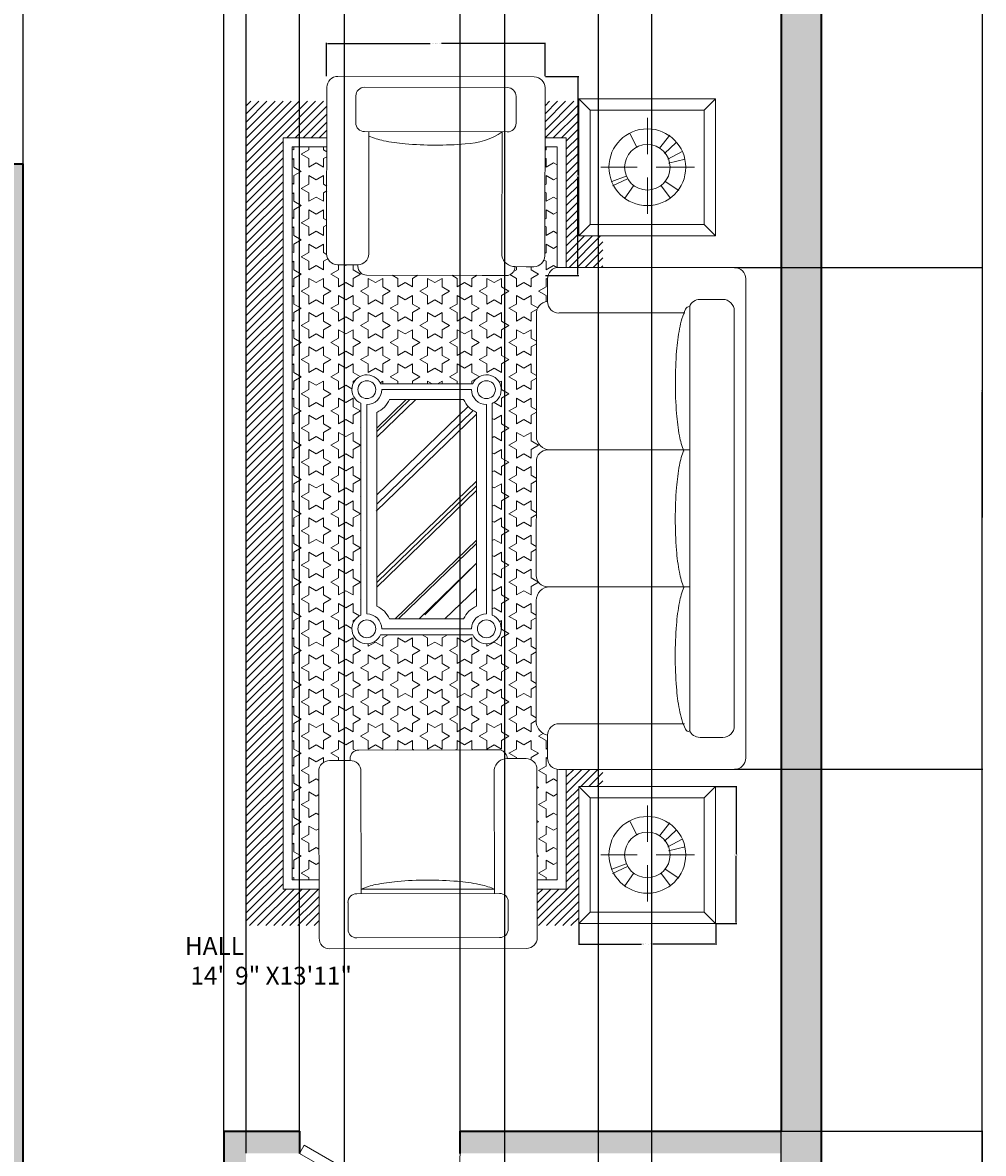
# Model space of a CAD drawing. Units: inches. Extents: x -29 to 404, y -32 to 761.
# Tile 4 of 5: x 189 to 404, y 193 to 447. Entities that reach past the tile are written whole.
import ezdxf

# ---------------------------------------------------------------- set-up
doc = ezdxf.new("R2010")
doc.units = ezdxf.units.IN
doc.header["$MEASUREMENT"] = 0
for name, color, linetype, lineweight in [('A-ANNO-DIMS', 2, 'Continuous', 18), ('A-AREA-IDEN', 7, 'Continuous', 18), ('A-FLOR-PATT', 9, 'Continuous', 13), ('A-FURN', 8, 'Continuous', 18), ('A-WALL', 7, 'Continuous', 35), ('doors', 40, 'Continuous', 20)]:
    doc.layers.add(name, color=color, linetype=linetype, lineweight=lineweight)
doc.layers.add('A-WALL-PATT', color=251, linetype='Continuous', lineweight=13, true_color=0x636466)
doc.styles.get("Standard").update_dxf_attribs({"font": 'arial.ttf'})
doc.dimstyles.get("Standard").update_dxf_attribs({"dimtxt": 0.18, "dimasz": 0.18, "dimexe": 0.18, "dimexo": 0.0625, "dimgap": 0.09, "dimtad": 0, "dimtih": 1, "dimtoh": 1, "dimdec": 4, "dimzin": 0, "dimdsep": 46, "dimtxsty": 'Standard', "dimcen": 0.09, "dimadec": 0, "dimazin": 0, "dimtfac": 1, "dimtdec": 4, "dimtofl": 0, "dimtmove": 0, "dimatfit": 3, "dimfxl": 1, "dimtolj": 1, "dimtzin": 0, "dimarcsym": 0})
pattern_1 = [(45, (602.1246, 1762.0968), (0.9050907, -0.9050907), [])]

# ---------------------------------------------------------------- blocks, each defined once
blk = doc.blocks.new('*U7')
for p, q in [((0, 0), (0, 100)), ((750, 0), (750, 100))]:
    blk.add_line(p, q)
blk.add_lwpolyline([(0, 0), (649.5, -375), (671.4, -337.1), (21.9, 37.9)], close=True)
blk.add_arc((0, 0), 750, 330, 0)
blk = doc.blocks.new('END-TABLE-HALL')
for p, q in [((0, 0), (0, 30.72)), ((0, 30.72), (30.72, 30.72)), ((2.56, 28.16), (0, 30.72)), ((28.16, 28.16), (30.72, 30.72)), ((30.72, 30.72), (30.72, 0)), ((2.56, 28.16), (28.16, 28.16)), ((2.56, 2.56), (2.56, 28.16)), ((28.16, 28.16), (28.16, 2.56)), ((15.4, 18.29), (15.4, 26.44)), ((12.94, 19.98), (11.56, 22.9)), ((18.16, 19.68), (20.47, 22.6)), ((19.24, 18.45), (21.85, 20.91)), ((20.01, 17.22), (23.23, 18.91)), ((4.95, 15.38), (13.09, 15.38)), ((17.4, 15.38), (26, 15.38)), ((20.16, 16.3), (23.85, 17.22)), ((10.64, 13.38), (7.41, 12.15)), ((10.94, 12.77), (7.56, 11.23)), ((15.4, 4.93), (15.4, 13.07)), ((12.33, 11.23), (10.33, 8.46)), ((18.47, 11.23), (20.62, 8.46)), ((19.39, 12.15), (22.46, 10.15)), ((2.56, 2.56), (0, 0)), ((28.16, 2.56), (2.56, 2.56)), ((28.16, 2.56), (30.72, 0)), ((30.72, 0), (0, 0))]:
    blk.add_line(p, q)
for radius in [8.61, 5.11]:
    blk.add_circle((15.4, 15.38), radius)
blk = doc.blocks.new('ARMCHAIR-HALL')
for p, q in [((8.97, 44.58), (35.98, 44.64)), ((34.86, 44.63), (40.72, 44.64)), ((2.43, 42.25), (7.02, 42.26)), ((7.02, 42.26), (7.03, 42.63)), ((44.98, 42.69), (42.28, 42.68)), ((44.74, 42.7), (46.49, 42.7)), ((0.07, 2.43), (0, 39.82)), ((9.51, 12.37), (9.46, 39.84)), ((39.38, 12.44), (39.33, 40.24)), ((49.01, 2.54), (48.93, 40.28)), ((6.56, 10.42), (6.57, 4.39)), ((8.5, 12.37), (40.53, 12.44)), ((42.49, 4.47), (42.48, 10.5)), ((2.51, 0), (46.58, 0.1)), ((8.52, 2.44), (40.55, 2.52))]:
    blk.add_line(p, q)
for centre, radius, start, end in [((8.97, 42.64), 1.95, 90.1148, 180.1148), ((40.17, 42.59), 2.11, 2.3345, 74.9758), ((2.43, 39.82), 2.43, 90.1148, 180.1148), ((7.03, 39.83), 2.43, 0.1148, 90.1148), ((42.21, 39.75), 2.93, 88.725, 170.3573), ((46.5, 40.27), 2.43, 0.1148, 90.1148), ((8.5, 10.42), 1.95, 90.1148, 180.1148), ((40.54, 10.5), 1.95, 0.1148, 90.1148), ((8.51, 4.39), 1.95, 180.1148, 270.1148), ((40.55, 4.47), 1.95, 270.1148, 0.1148), ((46.57, 2.53), 2.43, 270.1148, 0.1148), ((2.51, 2.43), 2.43, 180.1148, 270.1298)]:
    blk.add_arc(centre, radius, start, end)
blk = doc.blocks.new('*D17')
at = {"layer": 'A-ANNO-DIMS', "color": 0, "lineweight": -2, "transparency": 16777216}
for p, q in [((313.28, 244.96), (313.28, 240.23)), ((344, 244.96), (344, 240.23)), ((313.46, 240.41), (327.38, 240.41)), ((343.82, 240.41), (329.89, 240.41))]:
    blk.add_line(p, q, dxfattribs=at)
at = {"layer": 'A-ANNO-DIMS', "color": 0, "transparency": 16777216}
for points in [[(313.46, 240.44), (313.46, 240.38), (313.28, 240.41)], [(343.82, 240.44), (343.82, 240.38), (344, 240.41)]]:
    blk.add_solid(points, dxfattribs=at)
at = {"layer": 'Defpoints', "color": 0, "transparency": 16777216}
for p in [(313.28, 245.02), (344, 245.02), (344, 240.41)]:
    blk.add_point(p, dxfattribs=at)
at = {"layer": 'A-ANNO-DIMS', "color": 0, "transparency": 16777216, "insert": (328.64, 240.41), "char_height": 0.18, "attachment_point": 5}
blk.add_mtext('\\A1;END TABLE 31 TYP.', dxfattribs=at)
blk = doc.blocks.new('*D18')
at = {"layer": 'A-ANNO-DIMS', "color": 0, "lineweight": -2, "transparency": 16777216}
for p, q in [((344.06, 275.74), (348.78, 275.74)), ((348.6, 275.56), (348.6, 260.56)), ((348.6, 245.2), (348.6, 260.2)), ((344.06, 245.02), (348.78, 245.02))]:
    blk.add_line(p, q, dxfattribs=at)
at = {"layer": 'A-ANNO-DIMS', "color": 0, "transparency": 16777216}
for points in [[(348.57, 275.56), (348.63, 275.56), (348.6, 275.74)], [(348.57, 245.2), (348.63, 245.2), (348.6, 245.02)]]:
    blk.add_solid(points, dxfattribs=at)
at = {"layer": 'Defpoints', "color": 0, "transparency": 16777216}
for p in [(344, 275.74), (348.6, 275.74), (344, 245.02)]:
    blk.add_point(p, dxfattribs=at)
at = {"layer": 'A-ANNO-DIMS', "color": 0, "transparency": 16777216, "insert": (348.6, 260.38), "char_height": 0.18, "attachment_point": 5}
blk.add_mtext('\\A1;31 TYP.', dxfattribs=at)
blk = doc.blocks.new('*D21')
at = {"layer": 'A-ANNO-DIMS', "color": 0, "lineweight": -2, "transparency": 16777216}
for p, q in [((256.74, 435.12), (256.74, 442.59)), ((256.92, 442.41), (280.01, 442.41)), ((305.57, 442.41), (282.48, 442.41)), ((305.75, 435.12), (305.75, 442.59))]:
    blk.add_line(p, q, dxfattribs=at)
at = {"layer": 'A-ANNO-DIMS', "color": 0, "transparency": 16777216}
for points in [[(256.92, 442.44), (256.92, 442.38), (256.74, 442.41)], [(305.57, 442.44), (305.57, 442.38), (305.75, 442.41)]]:
    blk.add_solid(points, dxfattribs=at)
at = {"layer": 'Defpoints', "color": 0, "transparency": 16777216}
for p in [(305.75, 442.41), (256.74, 435.06), (305.75, 435.06)]:
    blk.add_point(p, dxfattribs=at)
at = {"layer": 'A-ANNO-DIMS', "color": 0, "transparency": 16777216, "insert": (281.25, 442.41), "char_height": 0.18, "attachment_point": 5}
blk.add_mtext('\\A1;ARMCHAIR 49 TYP.', dxfattribs=at)
blk = doc.blocks.new('*D22')
at = {"layer": 'A-ANNO-DIMS', "color": 0, "lineweight": -2, "transparency": 16777216}
for p, q in [((305.81, 435.06), (313.28, 435.06)), ((313.1, 434.88), (313.1, 412.92)), ((313.1, 390.6), (313.1, 412.56)), ((305.81, 390.42), (313.28, 390.42))]:
    blk.add_line(p, q, dxfattribs=at)
at = {"layer": 'A-ANNO-DIMS', "color": 0, "transparency": 16777216}
for points in [[(313.07, 434.88), (313.13, 434.88), (313.1, 435.06)], [(313.07, 390.6), (313.13, 390.6), (313.1, 390.42)]]:
    blk.add_solid(points, dxfattribs=at)
at = {"layer": 'Defpoints', "color": 0, "transparency": 16777216}
for p in [(305.75, 435.06), (305.75, 390.42), (313.1, 390.42)]:
    blk.add_point(p, dxfattribs=at)
at = {"layer": 'A-ANNO-DIMS', "color": 0, "transparency": 16777216, "insert": (313.1, 412.74), "char_height": 0.18, "attachment_point": 5}
blk.add_mtext('\\A1;45 TYP.', dxfattribs=at)
blk = doc.blocks.new('*D32')
at = {"layer": 'A-ANNO-DIMS', "color": 0, "lineweight": -2, "transparency": 16777216}
for p, q in [((367.74, 724.43), (403.91, 724.43)), ((403.73, 724.25), (403.73, 364.62)), ((403.73, 4.61), (403.73, 364.25)), ((367.74, 4.43), (403.91, 4.43))]:
    blk.add_line(p, q, dxfattribs=at)
at = {"layer": 'A-ANNO-DIMS', "color": 0, "transparency": 16777216}
for points in [[(403.7, 724.25), (403.76, 724.25), (403.73, 724.43)], [(403.7, 4.61), (403.76, 4.61), (403.73, 4.43)]]:
    blk.add_solid(points, dxfattribs=at)
at = {"layer": 'Defpoints', "color": 0, "transparency": 16777216}
for p in [(367.68, 724.43), (403.73, 724.43), (367.68, 4.43)]:
    blk.add_point(p, dxfattribs=at)
at = {"layer": 'A-ANNO-DIMS', "color": 0, "transparency": 16777216, "insert": (403.73, 364.43), "char_height": 0.18, "attachment_point": 5}
blk.add_mtext('\\A1;720', dxfattribs=at)
blk = doc.blocks.new('*D41')
at = {"layer": 'A-ANNO-DIMS', "color": 0, "lineweight": -2, "transparency": 16777216}
for p, q in [((250.68, 193.5), (250.68, 760.66)), ((250.86, 760.48), (268.46, 760.48)), ((286.5, 760.48), (268.9, 760.48)), ((286.68, 193.5), (286.68, 760.66))]:
    blk.add_line(p, q, dxfattribs=at)
at = {"layer": 'A-ANNO-DIMS', "color": 0, "transparency": 16777216}
for points in [[(250.86, 760.51), (250.86, 760.45), (250.68, 760.48)], [(286.5, 760.51), (286.5, 760.45), (286.68, 760.48)]]:
    blk.add_solid(points, dxfattribs=at)
at = {"layer": 'Defpoints', "color": 0, "transparency": 16777216}
for p in [(286.68, 760.48), (250.68, 193.43), (286.68, 193.43)]:
    blk.add_point(p, dxfattribs=at)
at = {"layer": 'A-ANNO-DIMS', "color": 0, "transparency": 16777216, "insert": (268.68, 760.48), "char_height": 0.18, "attachment_point": 5}
blk.add_mtext('\\A1;36', dxfattribs=at)
blk = doc.blocks.new('*D42')
at = {"layer": 'A-ANNO-DIMS', "color": 0, "lineweight": -2, "transparency": 16777216}
for p, q in [((238.68, 193.5), (238.68, 760.66)), ((238.86, 760.48), (244.47, 760.48)), ((250.5, 760.48), (244.89, 760.48)), ((250.68, 193.5), (250.68, 760.66))]:
    blk.add_line(p, q, dxfattribs=at)
at = {"layer": 'A-ANNO-DIMS', "color": 0, "transparency": 16777216}
for points in [[(238.86, 760.51), (238.86, 760.45), (238.68, 760.48)], [(250.5, 760.51), (250.5, 760.45), (250.68, 760.48)]]:
    blk.add_solid(points, dxfattribs=at)
at = {"layer": 'Defpoints', "color": 0, "transparency": 16777216}
for p in [(250.68, 760.48), (238.68, 193.43), (250.68, 193.43)]:
    blk.add_point(p, dxfattribs=at)
at = {"layer": 'A-ANNO-DIMS', "color": 0, "transparency": 16777216, "insert": (244.68, 760.48), "char_height": 0.18, "attachment_point": 5}
blk.add_mtext('\\A1;12', dxfattribs=at)
blk = doc.blocks.new('*D44')
at = {"layer": 'A-ANNO-DIMS', "color": 0, "lineweight": -2, "transparency": 16777216}
for p, q in [((188.68, 92.5), (188.68, 760.66)), ((188.86, 760.48), (210.95, 760.48)), ((233.5, 760.48), (211.4, 760.48)), ((233.68, 92.5), (233.68, 760.66))]:
    blk.add_line(p, q, dxfattribs=at)
at = {"layer": 'A-ANNO-DIMS', "color": 0, "transparency": 16777216}
for points in [[(188.86, 760.51), (188.86, 760.45), (188.68, 760.48)], [(233.5, 760.51), (233.5, 760.45), (233.68, 760.48)]]:
    blk.add_solid(points, dxfattribs=at)
at = {"layer": 'Defpoints', "color": 0, "transparency": 16777216}
for p in [(233.68, 760.48), (188.68, 92.43), (233.68, 92.43)]:
    blk.add_point(p, dxfattribs=at)
at = {"layer": 'A-ANNO-DIMS', "color": 0, "transparency": 16777216, "insert": (211.18, 760.48), "char_height": 0.18, "attachment_point": 5}
blk.add_mtext('\\A1;45', dxfattribs=at)
blk = doc.blocks.new('*D45')
at = {"layer": 'A-ANNO-DIMS', "color": 0, "lineweight": -2, "transparency": 16777216}
for p, q in [((329.68, 126.5), (329.68, 760.66)), ((329.86, 760.48), (343.96, 760.48)), ((358.5, 760.48), (344.4, 760.48)), ((358.68, 97.5), (358.68, 760.66))]:
    blk.add_line(p, q, dxfattribs=at)
at = {"layer": 'A-ANNO-DIMS', "color": 0, "transparency": 16777216}
for points in [[(329.86, 760.51), (329.86, 760.45), (329.68, 760.48)], [(358.5, 760.51), (358.5, 760.45), (358.68, 760.48)]]:
    blk.add_solid(points, dxfattribs=at)
at = {"layer": 'Defpoints', "color": 0, "transparency": 16777216}
for p in [(358.68, 760.48), (329.68, 126.43), (358.68, 97.43)]:
    blk.add_point(p, dxfattribs=at)
at = {"layer": 'A-ANNO-DIMS', "color": 0, "transparency": 16777216, "insert": (344.18, 760.48), "char_height": 0.18, "attachment_point": 5}
blk.add_mtext('\\A1;29', dxfattribs=at)
blk = doc.blocks.new('*D49')
at = {"layer": 'A-ANNO-DIMS', "color": 0, "lineweight": -2, "transparency": 16777216}
for p, q in [((348.24, 392.2), (403.91, 392.2)), ((403.73, 392.02), (403.73, 336.08)), ((403.73, 279.78), (403.73, 335.72)), ((348.24, 279.6), (403.91, 279.6))]:
    blk.add_line(p, q, dxfattribs=at)
at = {"layer": 'A-ANNO-DIMS', "color": 0, "transparency": 16777216}
for points in [[(403.7, 392.02), (403.76, 392.02), (403.73, 392.2)], [(403.7, 279.78), (403.76, 279.78), (403.73, 279.6)]]:
    blk.add_solid(points, dxfattribs=at)
at = {"layer": 'Defpoints', "color": 0, "transparency": 16777216}
for p in [(348.18, 392.2), (348.18, 279.6), (403.73, 279.6)]:
    blk.add_point(p, dxfattribs=at)
at = {"layer": 'A-ANNO-DIMS', "color": 0, "transparency": 16777216, "insert": (403.73, 335.9), "char_height": 0.18, "attachment_point": 5}
blk.add_mtext('\\A1;112.6', dxfattribs=at)
blk = doc.blocks.new('*D50')
at = {"layer": 'A-ANNO-DIMS', "color": 0, "lineweight": -2, "transparency": 16777216}
for p, q in [((260.68, 466.37), (260.68, -31.8)), ((296.68, 466.37), (296.68, -31.8)), ((260.86, -31.62), (278.46, -31.62)), ((296.5, -31.62), (278.9, -31.62))]:
    blk.add_line(p, q, dxfattribs=at)
at = {"layer": 'A-ANNO-DIMS', "color": 0, "transparency": 16777216}
for points in [[(260.86, -31.59), (260.86, -31.65), (260.68, -31.62)], [(296.5, -31.59), (296.5, -31.65), (296.68, -31.62)]]:
    blk.add_solid(points, dxfattribs=at)
at = {"layer": 'Defpoints', "color": 0, "transparency": 16777216}
for p in [(260.68, 466.43), (296.68, 466.43), (296.68, -31.62)]:
    blk.add_point(p, dxfattribs=at)
at = {"layer": 'A-ANNO-DIMS', "color": 0, "transparency": 16777216, "insert": (278.68, -31.62), "char_height": 0.18, "attachment_point": 5}
blk.add_mtext('\\A1;36', dxfattribs=at)
blk = doc.blocks.new('*D51')
at = {"layer": 'A-ANNO-DIMS', "color": 0, "lineweight": -2, "transparency": 16777216}
for p, q in [((296.68, 471.37), (296.68, -31.8)), ((317.68, 471.37), (317.68, -31.8)), ((296.86, -31.62), (306.97, -31.62)), ((317.5, -31.62), (307.38, -31.62))]:
    blk.add_line(p, q, dxfattribs=at)
at = {"layer": 'A-ANNO-DIMS', "color": 0, "transparency": 16777216}
for points in [[(296.86, -31.59), (296.86, -31.65), (296.68, -31.62)], [(317.5, -31.59), (317.5, -31.65), (317.68, -31.62)]]:
    blk.add_solid(points, dxfattribs=at)
at = {"layer": 'Defpoints', "color": 0, "transparency": 16777216}
for p in [(296.68, 471.43), (317.68, 471.43), (317.68, -31.62)]:
    blk.add_point(p, dxfattribs=at)
at = {"layer": 'A-ANNO-DIMS', "color": 0, "transparency": 16777216, "insert": (307.18, -31.62), "char_height": 0.18, "attachment_point": 5}
blk.add_mtext('\\A1;21', dxfattribs=at)
blk = doc.blocks.new('*D55')
at = {"layer": 'A-ANNO-DIMS', "color": 0, "lineweight": -2, "transparency": 16777216}
for p, q in [((358.74, 198.43), (403.91, 198.43)), ((403.73, 198.25), (403.73, 145.62)), ((403.73, 92.61), (403.73, 145.25)), ((358.74, 92.43), (403.91, 92.43))]:
    blk.add_line(p, q, dxfattribs=at)
at = {"layer": 'A-ANNO-DIMS', "color": 0, "transparency": 16777216}
for points in [[(403.7, 198.25), (403.76, 198.25), (403.73, 198.43)], [(403.7, 92.61), (403.76, 92.61), (403.73, 92.43)]]:
    blk.add_solid(points, dxfattribs=at)
at = {"layer": 'Defpoints', "color": 0, "transparency": 16777216}
for p in [(358.68, 198.43), (403.73, 198.43), (358.68, 92.43)]:
    blk.add_point(p, dxfattribs=at)
at = {"layer": 'A-ANNO-DIMS', "color": 0, "transparency": 16777216, "insert": (403.73, 145.43), "char_height": 0.18, "attachment_point": 5}
blk.add_mtext('\\A1;106', dxfattribs=at)

msp = doc.modelspace()

# ---------------------------------------------------------------- hatches: boundary and pattern name
at = {"layer": 'A-FLOR-PATT'}
h = msp.add_hatch(dxfattribs=at)
h.set_pattern_fill('ANSI31', color=256, scale=10.239932, angle=90, style=0)
h.set_pattern_definition(pattern_1)
h.paths.add_polyline_path([(256.807, 427.424), (256.794, 421.28), (247.004, 421.28), (247.004, 252.731), (255.044, 252.731), (255.056, 246.587), (240.86, 246.587), (240.86, 427.424)], flags=16)
h.paths.add_polyline_path([(256.811, 429.472), (256.807, 427.424), (240.86, 427.424), (240.86, 246.587), (255.056, 246.587), (255.06, 244.539), (238.812, 244.539), (238.812, 429.472)])
h = msp.add_hatch(dxfattribs=at)
h.set_pattern_fill('ANSI31', color=256, scale=10.239932, angle=90, style=0)
h.set_pattern_definition(pattern_1)
h.paths.add_polyline_path([(318.683, 399.301), (318.683, 392.213), (316.635, 392.214), (316.635, 399.301)])
h.paths.add_polyline_path([(316.635, 399.301), (316.635, 392.214), (310.491, 392.217), (310.491, 421.28), (305.726, 421.28), (305.738, 427.424), (313.276, 427.424), (313.276, 399.301)])
h.paths.add_polyline_path([(313.276, 429.472), (313.276, 427.424), (305.738, 427.424), (305.742, 429.472)])
h = msp.add_hatch(dxfattribs=at)
h.set_pattern_fill('STARS', color=256, scale=15.3599, angle=30, style=0)
h.paths.add_polyline_path([(249.052, 254.779), (255.04, 254.779), (254.991, 279.141), (255.002, 279.382), (255.037, 279.618), (255.095, 279.849), (255.174, 280.072), (255.275, 280.287), (255.397, 280.491), (255.539, 280.684), (255.7, 280.862), (255.878, 281.024), (256.07, 281.167), (256.273, 281.289), (256.488, 281.391), (256.711, 281.472), (256.941, 281.53), (257.178, 281.566), (257.418, 281.578), (262.012, 281.587), (262.017, 281.958), (262.026, 282.15), (262.054, 282.339), (262.1, 282.524), (262.164, 282.703), (262.245, 282.875), (262.342, 283.038), (262.455, 283.192), (262.584, 283.335), (262.727, 283.464), (262.88, 283.578), (263.043, 283.676), (263.215, 283.758), (263.393, 283.822), (263.578, 283.869), (263.767, 283.898), (263.959, 283.907), (290.975, 283.963), (295.709, 283.962), (295.709, 283.958), (295.873, 283.907), (296.031, 283.844), (296.324, 283.682), (296.585, 283.478), (296.811, 283.238), (296.996, 282.965), (297.137, 282.666), (297.23, 282.344), (297.258, 282.176), (297.272, 282.005), (299.969, 282.01), (301.485, 282.027), (301.734, 282.015), (301.975, 281.978), (302.208, 281.919), (302.432, 281.838), (302.645, 281.736), (302.845, 281.614), (303.033, 281.474), (303.206, 281.318), (303.363, 281.145), (303.504, 280.959), (303.626, 280.758), (303.729, 280.546), (303.811, 280.323), (303.871, 280.09), (303.909, 279.848), (303.922, 279.6), (303.971, 254.779), (308.443, 254.779), (308.443, 279.616), (308.358, 279.632), (308.115, 279.692), (307.88, 279.777), (307.654, 279.883), (307.44, 280.012), (307.237, 280.161), (307.049, 280.331), (306.879, 280.519), (306.73, 280.721), (306.601, 280.936), (306.494, 281.161), (306.41, 281.397), (306.349, 281.639), (306.312, 281.888), (306.299, 282.141), (306.297, 287.261), (306.044, 287.329), (305.799, 287.416), (305.565, 287.521), (305.341, 287.643), (305.128, 287.781), (304.928, 287.934), (304.74, 288.103), (304.566, 288.284), (304.407, 288.479), (304.262, 288.685), (304.134, 288.903), (304.022, 289.13), (303.928, 289.367), (303.852, 289.613), (303.795, 289.866), (303.758, 290.125), (303.77, 317.468), (303.786, 317.782), (303.832, 318.087), (303.908, 318.381), (304.012, 318.663), (304.141, 318.932), (304.295, 319.185), (304.472, 319.422), (304.67, 319.64), (304.889, 319.838), (305.125, 320.015), (305.379, 320.168), (305.647, 320.298), (305.929, 320.401), (306.224, 320.476), (306.529, 320.523), (306.843, 320.539), (306.331, 320.539), (306.078, 320.551), (305.829, 320.589), (305.587, 320.65), (305.351, 320.734), (305.126, 320.841), (304.911, 320.969), (304.709, 321.119), (304.521, 321.289), (304.351, 321.477), (304.202, 321.679), (304.073, 321.894), (303.967, 322.12), (303.882, 322.355), (303.822, 322.598), (303.784, 322.847), (303.772, 323.1), (303.782, 348.7), (303.796, 348.961), (303.834, 349.216), (303.898, 349.461), (303.984, 349.696), (304.092, 349.92), (304.22, 350.131), (304.367, 350.328), (304.533, 350.51), (304.715, 350.675), (304.912, 350.822), (305.123, 350.95), (305.347, 351.058), (305.582, 351.144), (305.827, 351.207), (306.082, 351.245), (306.343, 351.259), (306.855, 351.258), (306.552, 351.274), (306.253, 351.318), (305.962, 351.392), (305.68, 351.493), (305.409, 351.621), (305.151, 351.775), (304.909, 351.955), (304.683, 352.159), (304.479, 352.384), (304.3, 352.627), (304.146, 352.885), (304.018, 353.156), (303.917, 353.438), (303.844, 353.729), (303.799, 354.028), (303.785, 354.332), (303.796, 381.61), (303.779, 381.881), (303.789, 382.152), (303.828, 382.418), (303.893, 382.678), (303.984, 382.93), (304.101, 383.173), (304.242, 383.403), (304.408, 383.619), (304.596, 383.817), (304.801, 383.993), (305.022, 384.146), (305.257, 384.276), (305.504, 384.38), (305.761, 384.46), (306.026, 384.513), (306.297, 384.538), (306.299, 389.658), (306.312, 389.92), (306.351, 390.174), (306.414, 390.42), (306.501, 390.655), (306.608, 390.878), (306.737, 391.089), (306.884, 391.287), (307.049, 391.468), (307.231, 391.633), (307.428, 391.781), (307.64, 391.909), (307.863, 392.017), (308.099, 392.103), (308.344, 392.166), (308.443, 392.183), (308.443, 419.232), (305.722, 419.232), (305.673, 394.785), (305.66, 394.536), (305.622, 394.295), (305.562, 394.062), (305.48, 393.839), (305.377, 393.626), (305.255, 393.426), (305.114, 393.239), (304.957, 393.067), (304.784, 392.91), (304.597, 392.77), (304.396, 392.649), (304.183, 392.547), (303.959, 392.466), (303.726, 392.406), (303.485, 392.37), (303.236, 392.358), (301.481, 392.361), (299.023, 392.38), (299.009, 392.208), (298.981, 392.041), (298.888, 391.719), (298.747, 391.419), (298.562, 391.147), (298.337, 390.906), (298.075, 390.703), (297.782, 390.541), (297.624, 390.477), (297.46, 390.426), (291.601, 390.432), (265.71, 390.477), (265.518, 390.487), (265.329, 390.516), (265.144, 390.562), (264.966, 390.627), (264.794, 390.708), (264.631, 390.806), (264.478, 390.92), (264.335, 391.05), (264.207, 391.193), (264.093, 391.347), (263.996, 391.51), (263.915, 391.682), (263.851, 391.861), (263.805, 392.045), (263.778, 392.234), (263.768, 392.427), (263.763, 392.797), (263.768, 392.427), (263.763, 392.797), (259.169, 392.806), (258.929, 392.819), (258.693, 392.854), (258.462, 392.913), (258.239, 392.993), (258.025, 393.095), (257.821, 393.218), (257.629, 393.36), (257.451, 393.522), (257.29, 393.701), (257.148, 393.893), (257.026, 394.097), (256.925, 394.312), (256.846, 394.536), (256.788, 394.766), (256.753, 395.003), (256.742, 395.243), (256.79, 419.232), (249.052, 419.232)])
h.paths.add_polyline_path([(264.443, 361.718), (264.192, 361.839), (263.954, 361.979), (263.731, 362.136), (263.524, 362.31), (263.332, 362.499), (263.157, 362.701), (262.999, 362.917), (262.859, 363.144), (262.737, 363.381), (262.635, 363.628), (262.552, 363.883), (262.49, 364.145), (262.449, 364.412), (262.43, 364.685), (262.433, 364.96), (262.459, 365.238), (262.509, 365.513), (262.58, 365.779), (262.671, 366.036), (262.783, 366.283), (262.913, 366.518), (263.061, 366.741), (263.226, 366.951), (263.407, 367.147), (263.603, 367.328), (263.813, 367.493), (264.037, 367.642), (264.272, 367.772), (264.519, 367.883), (264.776, 367.975), (265.042, 368.046), (265.317, 368.095), (265.594, 368.122), (265.87, 368.125), (266.142, 368.106), (266.41, 368.065), (266.671, 368.003), (266.926, 367.92), (267.173, 367.817), (267.411, 367.696), (267.638, 367.556), (267.853, 367.398), (268.056, 367.222), (268.245, 367.031), (268.418, 366.823), (268.576, 366.6), (268.716, 366.363), (268.837, 366.112), (289.511, 366.112), (289.632, 366.363), (289.772, 366.6), (289.929, 366.823), (290.103, 367.031), (290.292, 367.222), (290.494, 367.398), (290.71, 367.556), (290.937, 367.696), (291.174, 367.817), (291.421, 367.92), (291.676, 368.003), (291.938, 368.065), (292.205, 368.106), (292.478, 368.125), (292.753, 368.122), (293.031, 368.095), (293.306, 368.046), (293.572, 367.975), (293.829, 367.883), (294.075, 367.772), (294.311, 367.642), (294.534, 367.493), (294.744, 367.328), (294.94, 367.147), (295.121, 366.951), (295.286, 366.741), (295.435, 366.518), (295.565, 366.283), (295.676, 366.036), (295.768, 365.779), (295.839, 365.513), (295.888, 365.238), (295.915, 364.96), (295.918, 364.685), (295.899, 364.412), (295.858, 364.145), (295.795, 363.883), (295.713, 363.628), (295.61, 363.381), (295.489, 363.144), (295.349, 362.917), (295.191, 362.701), (295.015, 362.499), (294.824, 362.31), (294.616, 362.136), (294.393, 361.979), (294.156, 361.839), (293.905, 361.718), (293.905, 314.192), (294.156, 314.071), (294.393, 313.931), (294.616, 313.774), (294.824, 313.6), (295.015, 313.411), (295.191, 313.209), (295.349, 312.993), (295.489, 312.766), (295.61, 312.529), (295.713, 312.282), (295.795, 312.027), (295.858, 311.765), (295.899, 311.498), (295.918, 311.225), (295.915, 310.95), (295.888, 310.672), (295.839, 310.397), (295.768, 310.131), (295.676, 309.874), (295.565, 309.628), (295.435, 309.392), (295.286, 309.169), (295.121, 308.959), (294.94, 308.763), (294.744, 308.582), (294.534, 308.417), (294.311, 308.268), (294.075, 308.138), (293.829, 308.027), (293.572, 307.935), (293.306, 307.864), (293.031, 307.815), (292.753, 307.788), (292.478, 307.785), (292.205, 307.804), (291.938, 307.845), (291.676, 307.908), (291.421, 307.99), (291.174, 308.093), (290.937, 308.214), (290.71, 308.354), (290.494, 308.512), (290.292, 308.688), (290.103, 308.879), (289.929, 309.087), (289.772, 309.31), (289.632, 309.547), (289.511, 309.798), (268.837, 309.798), (268.716, 309.547), (268.576, 309.31), (268.418, 309.087), (268.245, 308.879), (268.056, 308.688), (267.853, 308.512), (267.638, 308.354), (267.411, 308.214), (267.173, 308.093), (266.926, 307.99), (266.671, 307.908), (266.41, 307.845), (266.142, 307.804), (265.87, 307.785), (265.594, 307.788), (265.317, 307.815), (265.042, 307.864), (264.776, 307.935), (264.519, 308.027), (264.272, 308.138), (264.037, 308.268), (263.813, 308.417), (263.603, 308.582), (263.407, 308.763), (263.226, 308.959), (263.061, 309.169), (262.913, 309.392), (262.783, 309.628), (262.671, 309.874), (262.58, 310.131), (262.509, 310.397), (262.459, 310.672), (262.433, 310.95), (262.43, 311.225), (262.449, 311.498), (262.49, 311.765), (262.552, 312.027), (262.635, 312.282), (262.737, 312.529), (262.859, 312.766), (262.999, 312.993), (263.157, 313.209), (263.332, 313.411), (263.524, 313.6), (263.731, 313.774), (263.954, 313.931), (264.192, 314.071), (264.443, 314.192)], flags=0)
h = msp.add_hatch(dxfattribs=at)
h.set_pattern_fill('ANSI31', color=256, scale=10.23993, style=0)
h.paths.add_polyline_path([(303.992, 244.539), (313.276, 244.539), (313.276, 275.74), (318.683, 275.74), (318.683, 279.586), (310.491, 279.583), (310.491, 252.731), (303.976, 252.731)])
at = {"layer": 'A-WALL-PATT'}
h = msp.add_hatch(color=256, dxfattribs=at)
h.dxf.hatch_style = 1
h.paths.add_polyline_path([(188.678, 415.434), (183.678, 415.434), (183.678, 287.434), (180.678, 287.434), (180.678, 282.434), (183.678, 282.434), (183.678, 198.434), (57.678, 198.434), (57.678, 282.434), (144.678, 282.434), (144.678, 287.434), (16.678, 287.434), (16.678, 548.434), (144.678, 548.434, -0.1168354), (148.504, 564.585), (148.451, 564.616), (149.501, 566.434), (180.678, 548.434), (180.678, 543.434), (183.678, 543.434), (191.678, 543.434), (191.678, 548.434), (191.678, 553.634), (225.453, 573.134), (226.591, 571.164), (226.533, 571.131, -0.1168354), (230.678, 553.634), (230.678, 548.434), (358.678, 548.434), (358.678, 471.434), (322.678, 471.434), (322.678, 543.434), (358.678, 543.434), (358.678, 548.434), (230.678, 548.434), (230.678, 543.434), (233.678, 543.434), (252.678, 543.434), (252.678, 466.434), (260.678, 466.434), (260.678, 471.434), (257.678, 471.434), (257.678, 543.434), (317.678, 543.434), (317.678, 471.434), (296.678, 471.434), (296.678, 466.434), (358.678, 466.434), (358.678, 198.434), (286.678, 198.434), (286.678, 193.434), (358.678, 193.434), (358.678, 97.434), (238.678, 97.434), (238.678, 193.434), (250.678, 193.434), (250.678, 198.434), (233.678, 198.434), (233.678, 92.434), (358.678, 92.434), (358.678, 13.434), (296.678, 13.434), (296.678, 4.434), (367.678, 4.434), (367.678, 724.434), (7.678, 724.434), (7.678, 4.434), (188.678, 4.434), (188.678, 13.434), (188.678, 154.434), (183.678, 154.434), (183.678, 13.434), (49.651, 13.434), (48.286, 12.069), (46.92, 13.434), (16.678, 13.434), (16.678, 193.434), (183.678, 193.434), (183.678, 190.434), (188.678, 190.434)])
h.paths.add_polyline_path([(52.678, 282.434), (52.678, 198.434), (16.678, 198.434), (16.678, 282.434)], flags=16)

# ---------------------------------------------------------------- linework, layer by layer
at = {"layer": 'A-FLOR-PATT'}
for p, q in [((247.004, 421.28), (256.794, 421.28)), ((247.004, 252.731), (247.004, 421.28)), ((305.726, 421.28), (310.491, 421.28)), ((310.491, 421.28), (310.491, 392.217)), ((249.052, 254.779), (249.052, 419.232)), ((249.052, 419.232), (256.79, 419.232)), ((305.722, 419.232), (308.443, 419.232)), ((308.443, 419.232), (308.443, 392.183)), ((304.028, 383.044), (304.032, 383.039)), ((304.028, 383.044), (304.028, 383.03)), ((308.443, 279.616), (308.443, 254.779)), ((310.491, 279.583), (310.491, 252.731)), ((255.04, 254.779), (249.052, 254.779)), ((308.443, 254.779), (303.971, 254.779)), ((255.044, 252.731), (247.004, 252.731)), ((310.491, 252.731), (303.976, 252.731))]:
    msp.add_line(p, q, dxfattribs=at)
at = {"layer": 'A-FURN'}
for p, q in [((308.86, 392.217), (348.175, 392.202)), ((306.297, 384.538), (306.299, 389.658)), ((350.734, 282.159), (350.734, 389.641)), ((338.223, 383.666), (338.185, 288.209)), ((345.613, 385.037), (340.493, 385.039)), ((303.796, 381.61), (303.785, 354.332)), ((337.088, 382.007), (308.928, 382.018)), ((337.016, 381.966), (336.89, 381.966)), ((348.171, 382.476), (348.171, 289.321)), ((268.837, 366.112), (289.511, 366.112)), ((289.236, 364.784), (269.112, 364.784)), ((264.443, 314.192), (264.443, 361.718)), ((265.77, 361.443), (265.77, 314.467)), ((267.982, 354.102), (276.728, 362.573)), ((267.982, 355.366), (275.422, 362.573)), ((267.982, 356.151), (274.611, 362.573)), ((267.982, 341.165), (288.488, 361.027)), ((287.483, 362.573), (270.864, 362.573)), ((292.577, 314.467), (292.577, 361.443)), ((293.905, 361.718), (293.905, 314.192)), ((267.893, 337.535), (290.366, 359.3)), ((267.982, 339.115), (289.627, 360.079)), ((267.982, 359.69), (267.982, 316.22)), ((290.366, 316.22), (290.366, 359.69)), ((338.21, 351.246), (306.343, 351.259)), ((303.782, 348.7), (303.772, 323.1)), ((267.982, 322.61), (290.366, 344.29)), ((267.982, 321.491), (290.366, 343.171)), ((267.982, 320.484), (290.366, 342.164)), ((272.121, 313.337), (290.366, 331.009)), ((272.894, 313.337), (290.366, 330.26)), ((277.48, 313.337), (290.366, 325.818)), ((290.366, 325.855), (278.748, 314.237)), ((283.284, 313.337), (290.366, 320.196)), ((338.198, 320.526), (306.331, 320.539)), ((303.758, 290.125), (303.77, 317.468)), ((270.864, 313.337), (287.483, 313.337)), ((289.511, 309.798), (268.837, 309.798)), ((269.112, 311.126), (289.236, 311.126)), ((308.856, 289.822), (336.722, 289.833)), ((337.016, 289.833), (336.89, 289.833)), ((306.297, 287.261), (306.299, 282.141)), ((345.613, 286.762), (340.493, 286.76)), ((308.86, 279.582), (348.175, 279.598)), ((294.372, 252.731), (264.502, 252.731))]:
    msp.add_line(p, q, dxfattribs=at)
for centre in [(265.77, 364.784), (292.577, 364.784), (265.77, 311.126), (292.577, 311.126)]:
    msp.add_circle(centre, 2.015, dxfattribs=at)
for centre, radius, start, end in [((273.042, 437.764), 17.481, 247.14646, 258.35907), ((287.348, 435.435), 15.531, 271.88287, 304.40883), ((277.939, 461.533), 41.749, 258.35907, 265.05692), ((281.261, 499.937), 80.296, 265.05692, 274.71346), ((308.859, 389.657), 2.56, 89.97718, 179.97718), ((348.174, 389.642), 2.56, 359.97718, 89.97718), ((306.407, 381.912), 2.629, 92.4092, 186.6005), ((308.857, 384.537), 2.56, 179.97718, 269.97718), ((338.118, 382.492), 0.93, 90.40229, 155.84083), ((340.492, 382.479), 2.56, 89.97718, 158.38596), ((345.611, 382.477), 2.56, 359.97718, 89.97718), ((355.097, 374.876), 19.539, 155.84083, 169.46261), ((382.32, 369.812), 47.229, 169.46261, 175.58099), ((426.398, 366.406), 91.438, 175.58099, 184.37337), ((265.77, 364.784), 3.342, 23.39915, 246.60085), ((292.577, 364.784), 3.342, 293.39915, 156.60085), ((265.77, 364.784), 3.342, 270, 0), ((292.577, 364.784), 3.342, 180, 270), ((265.77, 364.784), 5.554, 293.47043, 336.52957), ((292.577, 364.784), 5.554, 203.47043, 246.52957), ((382.318, 363.035), 47.229, 184.37337, 190.49175), ((306.856, 354.33), 3.072, 179.97718, 269.97718), ((355.09, 357.992), 19.539, 190.49175, 201.01048), ((306.342, 348.699), 2.56, 89.97718, 179.97718), ((355.085, 344.244), 19.539, 158.94387, 169.46261), ((382.308, 339.18), 47.229, 169.46261, 175.58099), ((426.386, 335.774), 91.438, 175.58099, 184.37337), ((382.305, 332.402), 47.229, 184.37337, 190.49175), ((306.332, 323.099), 2.56, 179.97718, 269.97718), ((355.078, 327.36), 19.539, 190.49175, 201.01048), ((306.842, 317.467), 3.072, 89.97718, 179.97718), ((355.073, 313.445), 19.539, 158.94387, 169.46261), ((265.77, 311.126), 5.554, 23.47043, 66.52957), ((292.577, 311.126), 5.554, 113.47043, 156.52957), ((382.296, 308.381), 47.229, 169.46261, 175.58099), ((265.77, 311.126), 3.342, 113.39915, 336.60085), ((265.77, 311.126), 3.342, 0, 90), ((292.577, 311.126), 3.342, 90, 180), ((292.577, 311.126), 3.342, 203.39915, 66.60085), ((426.374, 304.975), 91.438, 175.58099, 184.37337), ((382.293, 301.603), 47.229, 184.37337, 190.49175), ((355.066, 296.561), 19.539, 190.49175, 204.11352), ((307.02, 290.459), 3.279, 185.84921, 257.25575), ((308.857, 287.262), 2.56, 90.02282, 180.02282), ((345.611, 289.322), 2.56, 270.02282, 0.02282), ((338.081, 288.959), 0.93, 204.11352, 269.72511), ((340.492, 289.32), 2.56, 201.61404, 270.02282), ((308.859, 282.142), 2.56, 180.02282, 270.02282), ((348.174, 282.158), 2.56, 270.02282, 0.02282), ((271.291, 236.62), 17.481, 101.64093, 112.85354), ((276.188, 212.851), 41.749, 94.94308, 101.64093), ((279.509, 174.448), 80.296, 85.28651, 94.94306), ((282.677, 212.864), 41.749, 78.58866, 85.28651), ((287.479, 236.653), 17.481, 67.72824, 78.58866)]:
    msp.add_arc(centre, radius, start, end, dxfattribs=at)
at = {"layer": 'A-WALL'}
for p, q in [((358.678, 466.434), (358.678, 198.434)), ((183.678, 415.434), (188.678, 415.434)), ((188.678, 190.434), (188.678, 415.434)), ((233.678, 198.434), (233.678, 92.434)), ((233.678, 198.434), (250.678, 198.434)), ((238.678, 198.434), (250.678, 198.434)), ((250.678, 198.434), (250.678, 193.434)), ((250.678, 198.434), (250.678, 195.934)), ((286.678, 198.434), (358.678, 198.434)), ((286.678, 193.434), (286.678, 198.434))]:
    msp.add_line(p, q, dxfattribs=at)
msp.add_lwpolyline([(188.678, 4.434), (7.678, 4.434), (7.678, 724.434), (367.678, 724.434), (367.678, 4.434), (296.678, 4.434)], dxfattribs=at)

# ---------------------------------------------------------------- block references
at = {"layer": 'A-FURN', "extrusion": (0, 0, -1), "zscale": -1, "rotation": 180}
msp.add_blockref('ARMCHAIR-HALL', (-256.742, 435.061), dxfattribs=at)
at = {"layer": 'A-FURN'}
for name, p in [('END-TABLE-HALL', (313.276, 399.301)), ('ARMCHAIR-HALL', (254.991, 239.324)), ('END-TABLE-HALL', (313.276, 245.02))]:
    msp.add_blockref(name, p, dxfattribs=at)
at = {"layer": 'doors', "xscale": 0.0479999999999998, "yscale": 0.0479999999999998, "zscale": 0.0479999999999998}
msp.add_blockref('*U7', (250.678, 193.434), dxfattribs=at)

# ---------------------------------------------------------------- texts
at = {"layer": 'A-AREA-IDEN', "insert": (224.992, 241.979), "char_height": 4, "attachment_point": 1}
msp.add_mtext_dynamic_manual_height_columns('HALL\\P 14\'  9" X13\'11"', width=80.5, gutter_width=1, heights=[0], dxfattribs=at)

# ---------------------------------------------------------------- dimensions: what is measured, and where the dimension line sits
at = {"layer": 'A-ANNO-DIMS'}
for base, p1, p2, picture, middle in [((233.678, 760.484), (188.678, 92.434), (233.678, 92.434), '*D44', (211.178, 760.484)), ((250.678, 760.484), (238.678, 193.434), (250.678, 193.434), '*D42', (244.678, 760.484)), ((286.678, 760.484), (250.678, 193.434), (286.678, 193.434), '*D41', (268.678, 760.484)), ((358.678, 760.484), (329.678, 126.434), (358.678, 97.434), '*D45', (344.178, 760.484)), ((317.678, -31.616), (296.678, 471.434), (317.678, 471.434), '*D51', (307.178, -31.616)), ((296.678, -31.616), (260.678, 466.434), (296.678, 466.434), '*D50', (278.678, -31.616))]:
    dim = msp.add_linear_dim(base=base, p1=p1, p2=p2, dimstyle='Standard', override={"dimdec": 0, "dimlfac": 1, "dimrnd": 0, "dimzin": 0, "dimdsep": 46, "dimlunit": 2}, dxfattribs=at)
    dim.commit()
    dim.dimension.update_dxf_attribs({"geometry": picture, "text_midpoint": middle})
for base, p1, p2, override, picture, middle in [((403.728, 724.434), (367.678, 4.434), (367.678, 724.434), {"dimdec": 0, "dimlfac": 1, "dimrnd": 0, "dimzin": 0, "dimdsep": 46, "dimlunit": 2}, '*D32', (403.728, 364.434)), ((403.728, 279.598), (348.175, 392.202), (348.175, 279.598), {"dimdec": 1, "dimlfac": 1, "dimrnd": 0, "dimzin": 0, "dimdsep": 46, "dimlunit": 2}, '*D49', (403.728, 335.9)), ((403.728, 198.434), (358.678, 92.434), (358.678, 198.434), {"dimdec": 0, "dimlfac": 1, "dimrnd": 0, "dimzin": 0, "dimdsep": 46, "dimlunit": 2}, '*D55', (403.728, 145.434))]:
    dim = msp.add_linear_dim(base=base, p1=p1, p2=p2, angle=90, dimstyle='Standard', override=override, dxfattribs=at)
    dim.commit()
    dim.dimension.update_dxf_attribs({"geometry": picture, "text_midpoint": middle})
for base, p1, p2, text, picture, middle in [((305.75, 442.413), (256.741, 435.062), (305.75, 435.062), 'ARMCHAIR <> TYP.', '*D21', (281.245, 442.413)), ((343.995, 240.412), (313.276, 245.02), (343.995, 245.02), 'END TABLE <> TYP.', '*D17', (328.635, 240.412))]:
    dim = msp.add_linear_dim(base=base, p1=p1, p2=p2, text=text, dimstyle='Standard', override={"dimdec": 0, "dimlfac": 1, "dimrnd": 0, "dimzin": 0, "dimdsep": 46, "dimlunit": 2}, dxfattribs=at)
    dim.commit()
    dim.dimension.update_dxf_attribs({"geometry": picture, "text_midpoint": middle})
for base, p1, p2, angle, picture, middle in [((313.101, 390.422), (305.75, 435.062), (305.75, 390.422), 270, '*D22', (313.101, 412.742)), ((348.603, 275.74), (343.995, 245.02), (343.995, 275.74), 90, '*D18', (348.603, 260.38))]:
    dim = msp.add_linear_dim(base=base, p1=p1, p2=p2, angle=angle, text='<> TYP.', dimstyle='Standard', override={"dimdec": 0, "dimlfac": 1, "dimrnd": 0, "dimzin": 0, "dimdsep": 46, "dimlunit": 2}, dxfattribs=at)
    dim.commit()
    dim.dimension.update_dxf_attribs({"geometry": picture, "text_midpoint": middle})

doc.saveas('drawing.dxf')
